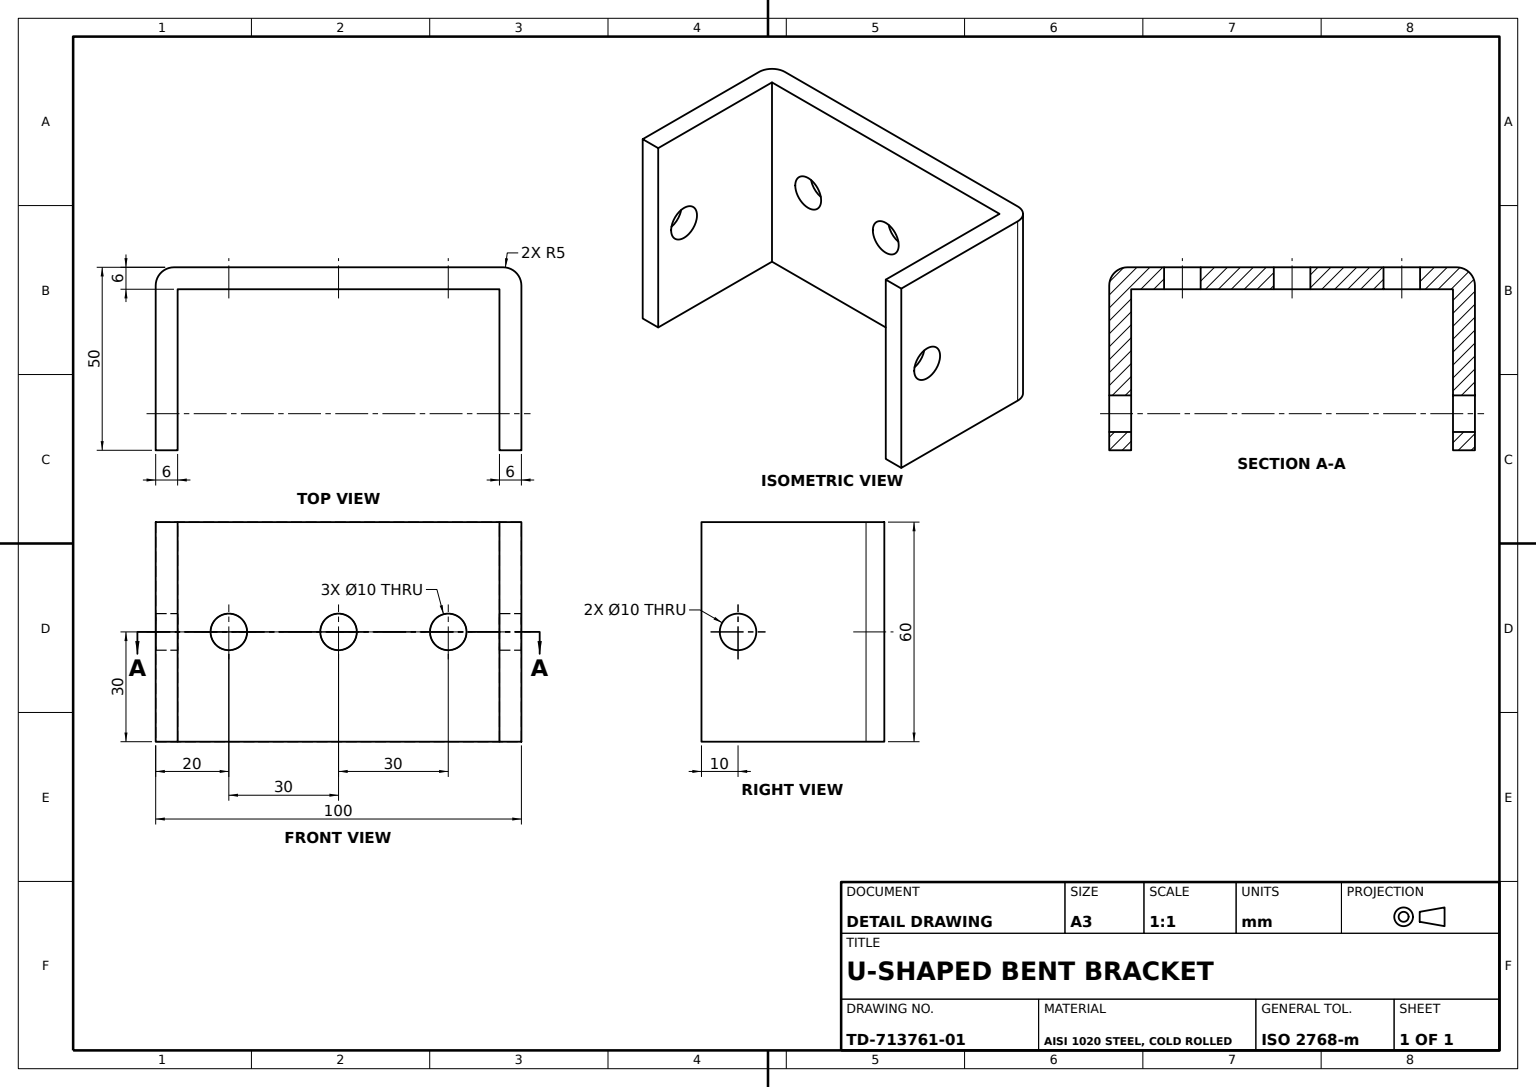
from build123d import *

# Parameters (mm, degrees)
CHANNEL_BODY_DEPTH      = 30
FLANGE_HOLES_SKETCH_R   = 5
FLANGE_HOLES_DEPTH      = 30
BACK_WALL_HOLES_REACH   = 117.758
BACK_WALL_HOLE_SKETCH_R = 5
CORNER_FILLETS_R5_R     = 5


with BuildPart() as part:
    # Channel Profile Sketch → Channel Body (new, symmetric)
    with BuildSketch(Plane(origin=(0, 0, 0), x_dir=(1, 0, 0), z_dir=(0, 1, 0))):
        Polygon((0, 0), (0, 50), (100, 50), (100, 0), (94, 0), (94, 44), (6, 44), (6, 0), align=None)
    extrude(amount=CHANNEL_BODY_DEPTH, both=True)

    # Flange Holes Sketch → Flange Holes (cut, symmetric)
    with BuildSketch(Plane(origin=(0, 0, -50), x_dir=(-1, 0, 0), z_dir=(0, 0, -1))):
        with Locations((-50, 0)):
            Circle(FLANGE_HOLES_SKETCH_R)
        with Locations((-20, 0)):
            Circle(FLANGE_HOLES_SKETCH_R)
        with Locations((-80, 0)):
            Circle(FLANGE_HOLES_SKETCH_R)
    extrude(amount=FLANGE_HOLES_DEPTH, both=True, mode=Mode.SUBTRACT)

    # Back Wall Holes: up to this face of the body (flat: up to its plane)
    back_wall_holes_end = Plane(part.part.faces().sort_by_distance((0, 0, -25))[0])
    # Back Wall Hole Sketch → Back Wall Holes (cut, up to the picked face)
    with BuildSketch(Plane(origin=(100, 0, 0), x_dir=(0, 0, -1), z_dir=(1, 0, 0)), mode=Mode.PRIVATE) as back_wall_holes_sk1:
        with Locations((10, 0)):
            Circle(BACK_WALL_HOLE_SKETCH_R)
    back_wall_holes_tool1 = split(extrude(back_wall_holes_sk1.sketch, amount=-BACK_WALL_HOLES_REACH, mode=Mode.PRIVATE), bisect_by=back_wall_holes_end, keep=Keep.BOTH, mode=Mode.PRIVATE)
    add(back_wall_holes_tool1.solids().sort_by(Axis((100, 0, -10), (-1, 0, 0)))[0], mode=Mode.SUBTRACT)

    # Corner Fillets R5
    corner_fillets_r5_edges = [part.edges().sort_by_distance(p)[0] for p in [
        (0, 0, -50),
        (100, 0, -50),
    ]]
    fillet(corner_fillets_r5_edges, radius=CORNER_FILLETS_R5_R)


solid = part.part
